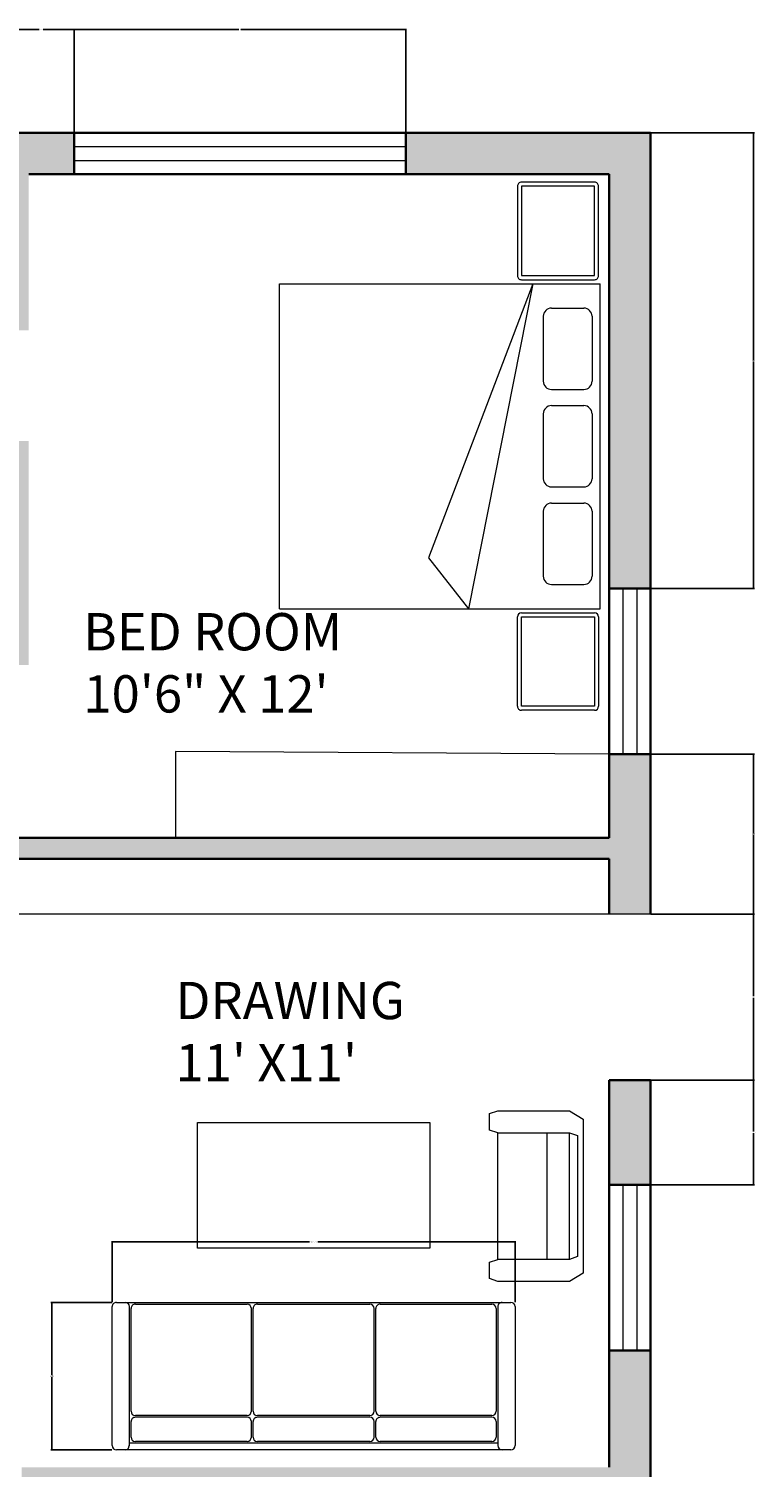
# Model space of a CAD drawing. Units: inches. Extents: x 2 to 2806, y 1095 to 1587.
# Tile 4 of 4: x 2648 to 2806, y 1275 to 1587. Entities that reach past the tile are written whole.
import ezdxf

# ---------------------------------------------------------------- set-up
doc = ezdxf.new("R2010")
doc.units = ezdxf.units.IN
for name, color, linetype, lineweight in [('A-ANNO-DIMS', 2, 'Continuous', 18), ('A-AREA-IDEN', 7, 'Continuous', 25), ('A-FLOR-CASE', 34, 'Continuous', 18), ('A-FURN', 8, 'Continuous', 18), ('A-GLAZ', 4, 'Continuous', 18), ('A-WALL', 7, 'Continuous', 35)]:
    doc.layers.add(name, color=color, linetype=linetype, lineweight=lineweight)
doc.layers.add('A-WALL-PATT', color=18, linetype='Continuous', lineweight=13, true_color=0x000000)
doc.styles.get("Standard").update_dxf_attribs({"font": 'arial.ttf'})
doc.dimstyles.get("Standard").update_dxf_attribs({"dimtxt": 0.18, "dimasz": 0.18, "dimexe": 0.18, "dimexo": 0.0625, "dimgap": 0.09, "dimtad": 0, "dimtih": 1, "dimtoh": 1, "dimdec": 4, "dimzin": 0, "dimdsep": 46, "dimtxsty": 'Standard', "dimcen": 0.09, "dimadec": 0, "dimazin": 0, "dimtfac": 1, "dimtdec": 4, "dimtofl": 0, "dimtmove": 0, "dimatfit": 3, "dimfxl": 1, "dimtolj": 1, "dimtzin": 0, "dimarcsym": 0})

# ---------------------------------------------------------------- blocks, each defined once
blk = doc.blocks.new('A$C793B20D3')
for p, q in [((0.625, 0), (0.625, 1.975)), ((2.625, 1.975), (0.625, 1.975)), ((2.625, 0), (2.625, 1.975)), ((2.675, 1.9655), (3.225, 1.9655)), ((0.575, 1.9405), (0.025, 1.9405)), ((0.025, 1.9405), (0.025, 1.4905)), ((0.575, 1.4905), (0.575, 1.9405)), ((0.775, 1.675), (0.775, 1.875)), ((0.825, 1.925), (1.225, 1.925)), ((1.275, 1.675), (1.275, 1.875)), ((1.375, 1.675), (1.375, 1.875)), ((1.425, 1.925), (1.825, 1.925)), ((1.875, 1.675), (1.875, 1.875)), ((1.975, 1.675), (1.975, 1.875)), ((2.025, 1.925), (2.425, 1.925)), ((2.475, 1.675), (2.475, 1.875)), ((2.65, 1.4905), (2.65, 1.9405)), ((3.25, 1.9405), (3.25, 1.4905)), ((0.825, 1.625), (1.225, 1.625)), ((1.425, 1.625), (1.825, 1.625)), ((2.025, 1.625), (2.425, 1.625)), ((0.6256, 1.5604), (2.3107, 0.9169)), ((0.6256, 1.5604), (2.625, 1.1646)), ((0.025, 1.4905), (0.575, 1.4905)), ((3.225, 1.4655), (2.675, 1.4655)), ((2.3107, 0.9169), (2.625, 1.1646)), ((2.625, 0), (0.625, 0))]:
    blk.add_line(p, q)
at = {"flags": 128}
blk.add_lwpolyline([(0, 1.9405), (0, 1.4905, 0.414214), (0.025, 1.4655), (0.575, 1.4655, 0.414214), (0.6, 1.4905), (0.6, 1.9405, 0.414214), (0.575, 1.9655), (0.025, 1.9655, 0.414214)], format="xyb", close=True, dxfattribs=at)
blk.add_lwpolyline([(3.225, 1.9405), (3.225, 1.4905), (2.675, 1.4905), (2.675, 1.9405)], close=True)
for centre, radius, start, end in [((2.675, 1.9405), 0.025, 90, 180), ((3.225, 1.9405), 0.025, 0, 90), ((0.825, 1.875), 0.05, 90, 180), ((1.225, 1.875), 0.05, 0, 90), ((1.425, 1.875), 0.05, 90, 180), ((1.825, 1.875), 0.05, 0, 90), ((2.025, 1.875), 0.05, 90, 180), ((2.425, 1.875), 0.05, 0, 90), ((0.825, 1.675), 0.05, 180, 270), ((1.225, 1.675), 0.05, 270, 0), ((1.425, 1.675), 0.05, 180, 270), ((1.825, 1.675), 0.05, 270, 0), ((2.025, 1.675), 0.05, 180, 270), ((2.425, 1.675), 0.05, 270, 0), ((2.675, 1.4905), 0.025, 180, 270), ((3.225, 1.4905), 0.025, 270, 0)]:
    blk.add_arc(centre, radius, start, end)
blk = doc.blocks.new('A$C0BA509B0')
for p, q in [((0.025, 0.86), (2.325, 0.86)), ((2.25, 0.8385), (2.25, 0.0224)), ((0, 0.025), (0, 0.835)), ((0.1, 0.0219), (0.1, 0.8375)), ((0.1, 0.82), (2.25, 0.82)), ((0.11, 0.695), (0.11, 0.785)), ((0.135, 0.81), (0.7866, 0.81)), ((0.8116, 0.785), (0.8116, 0.695)), ((0.8216, 0.785), (0.8216, 0.695)), ((0.8466, 0.81), (1.5033, 0.81)), ((1.5283, 0.785), (1.5283, 0.695)), ((1.5383, 0.785), (1.5383, 0.695)), ((1.5633, 0.81), (2.215, 0.81)), ((2.24, 0.785), (2.24, 0.695)), ((2.35, 0.835), (2.35, 0.025)), ((0.11, 0.035), (0.11, 0.635)), ((0.135, 0.67), (0.7866, 0.67)), ((0.135, 0.66), (0.7866, 0.66)), ((0.8116, 0.635), (0.8116, 0.035)), ((0.8216, 0.635), (0.8216, 0.035)), ((0.8466, 0.67), (1.5033, 0.67)), ((0.8466, 0.66), (1.5033, 0.66)), ((1.5283, 0.635), (1.5283, 0.035)), ((1.5383, 0.635), (1.5383, 0.035)), ((1.5633, 0.67), (2.215, 0.67)), ((1.5633, 0.66), (2.215, 0.66)), ((2.24, 0.635), (2.24, 0.035)), ((0.7866, 0.01), (0.135, 0.01)), ((1.5033, 0.01), (0.8466, 0.01)), ((2.215, 0.01), (1.5633, 0.01)), ((2.325, 0), (0.025, 0))]:
    blk.add_line(p, q)
for centre, start, end in [((0.025, 0.835), 90, 180), ((0.0751, 0.835), 0, 90), ((2.2752, 0.835), 90, 180), ((2.325, 0.835), 0, 90), ((0.135, 0.785), 90, 180), ((0.7866, 0.785), 0, 90), ((0.8466, 0.785), 90, 180), ((1.5033, 0.785), 0, 90), ((1.5633, 0.785), 90, 180), ((2.215, 0.785), 0, 90), ((0.135, 0.695), 180, 270), ((0.7866, 0.695), 270, 0), ((0.8466, 0.695), 180, 270), ((1.5033, 0.695), 270, 0), ((1.5633, 0.695), 180, 270), ((2.215, 0.695), 270, 0), ((0.135, 0.635), 90, 180), ((0.7866, 0.635), 0, 90), ((0.8466, 0.635), 90, 180), ((1.5033, 0.635), 0, 90), ((1.5633, 0.635), 90, 180), ((2.215, 0.635), 0, 90), ((0.025, 0.025), 180, 270), ((0.0751, 0.025), 270, 0), ((0.135, 0.035), 180, 270), ((0.7866, 0.035), 270, 0), ((0.8466, 0.035), 180, 270), ((1.5033, 0.035), 270, 0), ((1.5633, 0.035), 180, 270), ((2.215, 0.035), 270, 0), ((2.2749, 0.025), 180, 270), ((2.325, 0.025), 270, 0)]:
    blk.add_arc(centre, 0.025, start, end)
blk = doc.blocks.new('A$C61201922')
for p, q in [((0, 0.737), (0.076, 0.864)), ((0.076, 0.864), (1.499, 0.864)), ((0.203, 0.737), (0.229, 0.813)), ((0.229, 0.813), (1.346, 0.813)), ((1.346, 0.813), (1.372, 0.737)), ((1.499, 0.864), (1.575, 0.737)), ((0, 0.076), (0, 0.737)), ((0.203, 0.076), (0.203, 0.737)), ((1.372, 0.737), (0.203, 0.737)), ((1.372, 0.737), (1.372, 0.076)), ((1.575, 0.737), (1.575, 0.076)), ((1.372, 0.533), (0.203, 0.533)), ((0.025, 0), (0, 0.076)), ((0.178, 0), (0.025, 0)), ((0.203, 0.076), (0.178, 0)), ((1.372, 0.076), (0.203, 0.076)), ((1.397, 0), (1.372, 0.076)), ((1.549, 0), (1.397, 0)), ((1.575, 0.076), (1.549, 0))]:
    blk.add_line(p, q)
blk = doc.blocks.new('WIN-GLAZ-36x9')
for p, q in [((0, 3), (36, 3)), ((0, 0), (36, 0))]:
    blk.add_line(p, q)
blk = doc.blocks.new('TABLE-COFFEE-RECT')
blk.add_lwpolyline([(0, 27.27), (50.38, 27.27), (50.38, 0), (0, 0), (0, 27.27)])
blk = doc.blocks.new('*D34')
at = {"layer": 'A-ANNO-DIMS', "color": 0, "lineweight": -2, "transparency": 16777216}
for p, q in [((2666.26, 1310.54), (2666.26, 1323.77)), ((2666.44, 1323.59), (2709.09, 1323.59)), ((2753.54, 1323.59), (2710.9, 1323.59)), ((2753.72, 1310.54), (2753.72, 1323.77))]:
    blk.add_line(p, q, dxfattribs=at)
at = {"layer": 'A-ANNO-DIMS', "color": 0, "transparency": 16777216}
for points in [[(2666.44, 1323.62), (2666.44, 1323.56), (2666.26, 1323.59)], [(2753.54, 1323.62), (2753.54, 1323.56), (2753.72, 1323.59)]]:
    blk.add_solid(points, dxfattribs=at)
at = {"layer": 'Defpoints', "color": 0, "transparency": 16777216}
for p in [(2666.26, 1323.59), (2666.26, 1310.47), (2753.72, 1310.47)]:
    blk.add_point(p, dxfattribs=at)
at = {"layer": 'A-ANNO-DIMS', "color": 0, "transparency": 16777216, "insert": (2709.99, 1323.59), "char_height": 0.18, "attachment_point": 5}
blk.add_mtext('\\A1;SOFA 87 TYP.', dxfattribs=at)
blk = doc.blocks.new('*D35')
at = {"layer": 'A-ANNO-DIMS', "color": 0, "lineweight": -2, "transparency": 16777216}
for p, q in [((2666.2, 1310.47), (2652.96, 1310.47)), ((2653.14, 1310.29), (2653.14, 1294.65)), ((2653.14, 1278.65), (2653.14, 1294.29)), ((2666.2, 1278.47), (2652.96, 1278.47))]:
    blk.add_line(p, q, dxfattribs=at)
at = {"layer": 'A-ANNO-DIMS', "color": 0, "transparency": 16777216}
for points in [[(2653.11, 1310.29), (2653.17, 1310.29), (2653.14, 1310.47)], [(2653.11, 1278.65), (2653.17, 1278.65), (2653.14, 1278.47)]]:
    blk.add_solid(points, dxfattribs=at)
at = {"layer": 'Defpoints', "color": 0, "transparency": 16777216}
for p in [(2666.26, 1310.47), (2653.14, 1278.47), (2666.26, 1278.47)]:
    blk.add_point(p, dxfattribs=at)
at = {"layer": 'A-ANNO-DIMS', "color": 0, "transparency": 16777216, "insert": (2653.14, 1294.47), "char_height": 0.18, "attachment_point": 5}
blk.add_mtext('\\A1;32 TYP.', dxfattribs=at)
blk = doc.blocks.new('*D58')
at = {"layer": 'A-ANNO-DIMS', "color": 0, "lineweight": -2, "transparency": 16777216}
for p, q in [((2783.21, 1564.21), (2805.68, 1564.21)), ((2805.5, 1564.03), (2805.5, 1514.97)), ((2805.5, 1465.54), (2805.5, 1514.61)), ((2783.21, 1465.36), (2805.68, 1465.36))]:
    blk.add_line(p, q, dxfattribs=at)
at = {"layer": 'A-ANNO-DIMS', "color": 0, "transparency": 16777216}
for points in [[(2805.47, 1564.03), (2805.53, 1564.03), (2805.5, 1564.21)], [(2805.47, 1465.54), (2805.53, 1465.54), (2805.5, 1465.36)]]:
    blk.add_solid(points, dxfattribs=at)
at = {"layer": 'Defpoints', "color": 0, "transparency": 16777216}
for p in [(2783.14, 1564.21), (2805.5, 1564.21), (2783.14, 1465.36)]:
    blk.add_point(p, dxfattribs=at)
at = {"layer": 'A-ANNO-DIMS', "color": 0, "transparency": 16777216, "insert": (2805.5, 1514.79), "char_height": 0.18, "attachment_point": 5}
blk.add_mtext('\\A1;98.85', dxfattribs=at)
blk = doc.blocks.new('*D59')
at = {"layer": 'A-ANNO-DIMS', "color": 0, "lineweight": -2, "transparency": 16777216}
for p, q in [((2783.21, 1429.36), (2805.68, 1429.36)), ((2805.5, 1429.18), (2805.5, 1412.22)), ((2805.5, 1394.89), (2805.5, 1411.86)), ((2783.21, 1394.71), (2805.68, 1394.71))]:
    blk.add_line(p, q, dxfattribs=at)
at = {"layer": 'A-ANNO-DIMS', "color": 0, "transparency": 16777216}
for points in [[(2805.47, 1429.18), (2805.53, 1429.18), (2805.5, 1429.36)], [(2805.47, 1394.89), (2805.53, 1394.89), (2805.5, 1394.71)]]:
    blk.add_solid(points, dxfattribs=at)
at = {"layer": 'Defpoints', "color": 0, "transparency": 16777216}
for p in [(2783.14, 1429.36), (2805.5, 1429.36), (2783.14, 1394.71)]:
    blk.add_point(p, dxfattribs=at)
at = {"layer": 'A-ANNO-DIMS', "color": 0, "transparency": 16777216, "insert": (2805.5, 1412.04), "char_height": 0.18, "attachment_point": 5}
blk.add_mtext('\\A1;34.65', dxfattribs=at)
blk = doc.blocks.new('*D60')
at = {"layer": 'A-ANNO-DIMS', "color": 0, "lineweight": -2, "transparency": 16777216}
for p, q in [((2783.21, 1394.71), (2805.68, 1394.71)), ((2805.5, 1394.53), (2805.5, 1376.9)), ((2805.5, 1358.89), (2805.5, 1376.53)), ((2783.21, 1358.71), (2805.68, 1358.71))]:
    blk.add_line(p, q, dxfattribs=at)
at = {"layer": 'A-ANNO-DIMS', "color": 0, "transparency": 16777216}
for points in [[(2805.47, 1394.53), (2805.53, 1394.53), (2805.5, 1394.71)], [(2805.47, 1358.89), (2805.53, 1358.89), (2805.5, 1358.71)]]:
    blk.add_solid(points, dxfattribs=at)
at = {"layer": 'Defpoints', "color": 0, "transparency": 16777216}
for p in [(2783.14, 1394.71), (2805.5, 1394.71), (2783.14, 1358.71)]:
    blk.add_point(p, dxfattribs=at)
at = {"layer": 'A-ANNO-DIMS', "color": 0, "transparency": 16777216, "insert": (2805.5, 1376.71), "char_height": 0.18, "attachment_point": 5}
blk.add_mtext('\\A1;36', dxfattribs=at)
blk = doc.blocks.new('*D61')
at = {"layer": 'A-ANNO-DIMS', "color": 0, "lineweight": -2, "transparency": 16777216}
for p, q in [((2783.21, 1358.71), (2805.68, 1358.71)), ((2805.5, 1358.53), (2805.5, 1347.54)), ((2805.5, 1336.18), (2805.5, 1347.17)), ((2783.21, 1336), (2805.68, 1336))]:
    blk.add_line(p, q, dxfattribs=at)
at = {"layer": 'A-ANNO-DIMS', "color": 0, "transparency": 16777216}
for points in [[(2805.47, 1358.53), (2805.53, 1358.53), (2805.5, 1358.71)], [(2805.47, 1336.18), (2805.53, 1336.18), (2805.5, 1336)]]:
    blk.add_solid(points, dxfattribs=at)
at = {"layer": 'Defpoints', "color": 0, "transparency": 16777216}
for p in [(2783.14, 1358.71), (2805.5, 1358.71), (2783.14, 1336)]:
    blk.add_point(p, dxfattribs=at)
at = {"layer": 'A-ANNO-DIMS', "color": 0, "transparency": 16777216, "insert": (2805.5, 1347.36), "char_height": 0.18, "attachment_point": 5}
blk.add_mtext('\\A1;22.713', dxfattribs=at)
blk = doc.blocks.new('*D65')
at = {"layer": 'A-ANNO-DIMS', "color": 0, "lineweight": -2, "transparency": 16777216}
for p, q in [((2643.64, 1564.28), (2643.64, 1586.75)), ((2643.82, 1586.57), (2650.37, 1586.57)), ((2657.82, 1586.57), (2651.28, 1586.57)), ((2658, 1564.28), (2658, 1586.75))]:
    blk.add_line(p, q, dxfattribs=at)
at = {"layer": 'A-ANNO-DIMS', "color": 0, "transparency": 16777216}
for points in [[(2643.82, 1586.6), (2643.82, 1586.54), (2643.64, 1586.57)], [(2657.82, 1586.6), (2657.82, 1586.54), (2658, 1586.57)]]:
    blk.add_solid(points, dxfattribs=at)
at = {"layer": 'Defpoints', "color": 0, "transparency": 16777216}
for p in [(2658, 1586.57), (2643.64, 1564.21), (2658, 1564.21)]:
    blk.add_point(p, dxfattribs=at)
at = {"layer": 'A-ANNO-DIMS', "color": 0, "transparency": 16777216, "insert": (2650.82, 1586.57), "char_height": 0.18, "attachment_point": 5}
blk.add_mtext('\\A1;14.357', dxfattribs=at)
blk = doc.blocks.new('*D66')
at = {"layer": 'A-ANNO-DIMS', "color": 0, "lineweight": -2, "transparency": 16777216}
for p, q in [((2658, 1564.28), (2658, 1586.75)), ((2658.18, 1586.57), (2693.78, 1586.57)), ((2729.82, 1586.57), (2694.22, 1586.57)), ((2730, 1564.28), (2730, 1586.75))]:
    blk.add_line(p, q, dxfattribs=at)
at = {"layer": 'A-ANNO-DIMS', "color": 0, "transparency": 16777216}
for points in [[(2658.18, 1586.6), (2658.18, 1586.54), (2658, 1586.57)], [(2729.82, 1586.6), (2729.82, 1586.54), (2730, 1586.57)]]:
    blk.add_solid(points, dxfattribs=at)
at = {"layer": 'Defpoints', "color": 0, "transparency": 16777216}
for p in [(2730, 1586.57), (2658, 1564.21), (2730, 1564.21)]:
    blk.add_point(p, dxfattribs=at)
at = {"layer": 'A-ANNO-DIMS', "color": 0, "transparency": 16777216, "insert": (2694, 1586.57), "char_height": 0.18, "attachment_point": 5}
blk.add_mtext('\\A1;72', dxfattribs=at)

msp = doc.modelspace()

# ---------------------------------------------------------------- hatches: boundary and pattern name
at = {"layer": 'A-WALL-PATT'}
h = msp.add_hatch(color=256, dxfattribs=at)
h.dxf.hatch_style = 1
h.paths.add_polyline_path([(2444, 1564.2135), (2385.6427, 1564.2135), (2385.6427, 1465.2135), (2394.6427, 1465.2135), (2394.6427, 1555.2135), (2444, 1555.2135)])
h.paths.add_polyline_path([(2540, 1564.2135), (2480, 1564.2135), (2480, 1555.2135), (2514.6427, 1555.2135), (2514.6427, 1448.7135), (2550.1001, 1448.7135), (2550.1001, 1453.2135), (2519.1427, 1453.2135), (2519.1427, 1555.2135), (2540, 1555.2135)])
h.paths.add_polyline_path([(2619.6427, 1564.2135), (2564, 1564.2135), (2564, 1555.2135), (2579.1427, 1555.2135), (2579.1427, 1453.2135), (2577.7846, 1453.2135), (2577.7846, 1448.7135), (2648.1427, 1448.7135), (2648.1427, 1497.3535), (2643.6427, 1497.3535), (2643.6427, 1453.2135), (2583.6427, 1453.2135), (2583.6427, 1555.2135), (2619.6427, 1555.2135)])
h.paths.add_polyline_path([(2658, 1564.2135), (2643.6427, 1564.2135), (2643.6427, 1555.2135), (2643.6427, 1521.3535), (2648.1427, 1521.3535), (2648.1427, 1555.2135), (2658, 1555.2135)])
h.paths.add_polyline_path([(2783.1427, 1564.2135), (2730, 1564.2135), (2730, 1555.2135), (2774.1427, 1555.2135), (2774.1427, 1465.3633), (2783.1427, 1465.3633)])
h.paths.add_polyline_path([(2783.1427, 1429.3633), (2774.1427, 1429.3633), (2774.1427, 1411.2135), (2610.5887, 1411.2135), (2610.5887, 1406.7135), (2774.1427, 1406.7135), (2774.1427, 1394.7135), (2783.1427, 1394.7135)])
h.paths.add_polyline_path([(2783.1427, 1358.7135), (2774.1427, 1358.7135), (2774.1427, 1336), (2783.1427, 1336)])
h.paths.add_polyline_path([(2783.1427, 1300), (2774.1427, 1300), (2774.1427, 1274.7135), (2646.5887, 1274.7135), (2646.5887, 1270.2135), (2774.1427, 1270.2135), (2774.1427, 1126.2135), (2750.1427, 1126.2135), (2750.1427, 1117.2135), (2783.1427, 1117.2135)])
h.paths.add_polyline_path([(2607.6427, 1126.2135), (2567.1427, 1126.2135), (2567.1427, 1117.2135), (2607.6427, 1117.2135)])
h.paths.add_polyline_path([(2714.1427, 1126.2135), (2643.6427, 1126.2135), (2643.6427, 1117.2135), (2714.1427, 1117.2135)])
h.paths.add_polyline_path([(2607.6427, 1270.2135), (2610.5887, 1270.2135), (2610.5887, 1274.7135), (2579.1427, 1274.7135), (2579.1427, 1270.2135), (2603.1427, 1270.2135), (2603.1427, 1232.7135), (2538.6427, 1232.7135), (2538.6427, 1126.2135), (2543.1427, 1126.2135), (2543.1427, 1228.2135), (2603.1427, 1228.2135), (2603.1427, 1189.2001), (2607.6427, 1189.2001)])
h.paths.add_polyline_path([(2543.1427, 1126.2135), (2514.6427, 1126.2135), (2514.6427, 1117.2135), (2543.1427, 1117.2135)], flags=17)
h.paths.add_polyline_path([(2418.6427, 1126.2135), (2394.6427, 1126.2135), (2394.6427, 1270.2135), (2418.6427, 1270.2135), (2543.1427, 1270.2135), (2543.1427, 1274.7135), (2411.1427, 1274.7135), (2411.1427, 1310), (2402.1427, 1310), (2402.1427, 1274.7135), (2385.6427, 1274.7135), (2385.6427, 1117.2135), (2418.6427, 1117.2135)])
h.paths.add_polyline_path([(2543.1427, 1411.2135), (2394.6427, 1411.2135), (2394.6427, 1429.2135), (2385.6427, 1429.2135), (2385.6427, 1406.7135), (2402.1427, 1406.7135), (2402.1427, 1370), (2411.1427, 1370), (2411.1427, 1406.7135), (2543.1427, 1406.7135)])

# ---------------------------------------------------------------- linework, layer by layer
at = {"layer": 'A-FLOR-CASE'}
for p, q in [((2774.1427, 1429.3633), (2680, 1430)), ((2680, 1430), (2680, 1411.2135)), ((2783.1427, 1394.7135), (2623.3219, 1394.7135))]:
    msp.add_line(p, q, dxfattribs=at)
at = {"layer": 'A-GLAZ'}
for p, q in [((2658, 1561.2135), (2730, 1561.2135)), ((2658, 1558.2135), (2730, 1558.2135))]:
    msp.add_line(p, q, dxfattribs=at)
at = {"layer": 'A-WALL'}
for p, q in [((2385.6427, 1564.2135), (2783.1427, 1564.2135)), ((2658, 1564.2135), (2658, 1555.2135)), ((2730, 1564.2135), (2730, 1555.2135)), ((2783.1427, 1564.2135), (2783.1427, 1394.7135)), ((2648.1427, 1555.2135), (2774.1427, 1555.2135)), ((2774.1427, 1555.2135), (2774.1427, 1411.2135)), ((2774.1427, 1465.3633), (2783.1427, 1465.3633)), ((2774.1427, 1429.3633), (2783.1427, 1429.3633)), ((2610.5887, 1411.2135), (2774.1427, 1411.2135)), ((2610.5887, 1406.7135), (2774.1427, 1406.7135)), ((2774.1427, 1406.7135), (2774.1427, 1394.7135)), ((2774.1427, 1406.7135), (2774.1427, 1394.7135)), ((2783.1427, 1358.7135), (2774.1427, 1358.7135)), ((2774.1427, 1358.7135), (2774.1427, 1274.7135)), ((2783.1427, 1358.7135), (2783.1427, 1117.2135)), ((2774.1427, 1336), (2783.1427, 1336)), ((2774.1427, 1300), (2783.1427, 1300))]:
    msp.add_line(p, q, dxfattribs=at)

# ---------------------------------------------------------------- block references
at = {"layer": 'A-FURN'}
for name, p, xscale, yscale, zscale, rotation in [('A$C793B20D3', (2702.5852, 1553.4683), 35.25, 35.25, 35.25, 270), ('A$C61201922', (2748.2104, 1352.029), 23.48594063424203, 23.48594063424203, 23.48594063424203, 270), ('A$C0BA509B0', (2753.7218, 1310.4747), 37.21767998259284, 37.21767998259284, 37.21767998259284, 180)]:
    msp.add_blockref(name, p, dxfattribs=dict(at, xscale=xscale, yscale=yscale, zscale=zscale, rotation=rotation))
msp.add_blockref('TABLE-COFFEE-RECT', (2684.811, 1322.2607), dxfattribs=at)
at = {"layer": 'A-GLAZ', "rotation": 270.0000000000014}
for p in [(2777.1427, 1465.3633), (2777.1427, 1336)]:
    msp.add_blockref('WIN-GLAZ-36x9', p, dxfattribs=at)

# ---------------------------------------------------------------- texts
at = {"layer": 'A-AREA-IDEN', "insert": (2660, 1460), "char_height": 8.089392, "width": 95.977856, "attachment_point": 1}
msp.add_mtext('BED ROOM\\P10\'6" X 12\'', dxfattribs=at)
at = {"layer": 'A-AREA-IDEN', "insert": (2680, 1380), "char_height": 8.08939, "attachment_point": 1}
msp.add_mtext("DRAWING\\P11' X11'", dxfattribs=at)

# ---------------------------------------------------------------- dimensions: what is measured, and where the dimension line sits
at = {"layer": 'A-ANNO-DIMS'}
for base, p1, p2, override, picture, middle in [((2658, 1586.5735), (2643.6427, 1564.2135), (2658, 1564.2135), {"dimdec": 3, "dimlfac": 1, "dimrnd": 0, "dimzin": 0, "dimdsep": 46, "dimlunit": 2}, '*D65', (2650.8213, 1586.5735)), ((2730, 1586.5735), (2658, 1564.2135), (2730, 1564.2135), {"dimdec": 0, "dimlfac": 1, "dimrnd": 0, "dimzin": 0, "dimdsep": 46, "dimlunit": 2}, '*D66', (2694, 1586.5735))]:
    dim = msp.add_linear_dim(base=base, p1=p1, p2=p2, dimstyle='Standard', override=override, dxfattribs=at)
    dim.commit()
    dim.dimension.update_dxf_attribs({"geometry": picture, "text_midpoint": middle})
for base, p1, p2, override, picture, middle in [((2805.5027, 1564.2135), (2783.1427, 1465.3633), (2783.1427, 1564.2135), {"dimdec": 2, "dimlfac": 1, "dimrnd": 0, "dimzin": 0, "dimdsep": 46, "dimlunit": 2}, '*D58', (2805.5027, 1514.7884)), ((2805.5027, 1429.3633), (2783.1427, 1394.7135), (2783.1427, 1429.3633), {"dimdec": 2, "dimlfac": 1, "dimrnd": 0, "dimzin": 0, "dimdsep": 46, "dimlunit": 2}, '*D59', (2805.5027, 1412.0384)), ((2805.5027, 1394.7135), (2783.1427, 1358.7135), (2783.1427, 1394.7135), {"dimdec": 0, "dimlfac": 1, "dimrnd": 0, "dimzin": 0, "dimdsep": 46, "dimlunit": 2}, '*D60', (2805.5027, 1376.7135)), ((2805.50269, 1358.71345), (2783.14269, 1336), (2783.14269, 1358.71345), {"dimdec": 3, "dimlfac": 1, "dimrnd": 0, "dimzin": 0, "dimdsep": 46, "dimlunit": 2}, '*D61', (2805.50269, 1347.35673))]:
    dim = msp.add_linear_dim(base=base, p1=p1, p2=p2, angle=90, dimstyle='Standard', override=override, dxfattribs=at)
    dim.commit()
    dim.dimension.update_dxf_attribs({"geometry": picture, "text_midpoint": middle})
for base, p1, p2, angle, text, picture, middle in [((2666.2602, 1323.5939), (2753.7218, 1310.4747), (2666.2602, 1310.4747), 180, 'SOFA <> TYP.', '*D34', (2709.991, 1323.5939)), ((2653.141, 1278.4675), (2666.2602, 1310.4747), (2666.2602, 1278.4675), 270, '<> TYP.', '*D35', (2653.141, 1294.4711))]:
    dim = msp.add_linear_dim(base=base, p1=p1, p2=p2, angle=angle, text=text, dimstyle='Standard', override={"dimdec": 0, "dimlfac": 1, "dimrnd": 0, "dimzin": 0, "dimdsep": 46, "dimlunit": 2}, dxfattribs=at)
    dim.commit()
    dim.dimension.update_dxf_attribs({"geometry": picture, "text_midpoint": middle})

doc.saveas('drawing.dxf')
